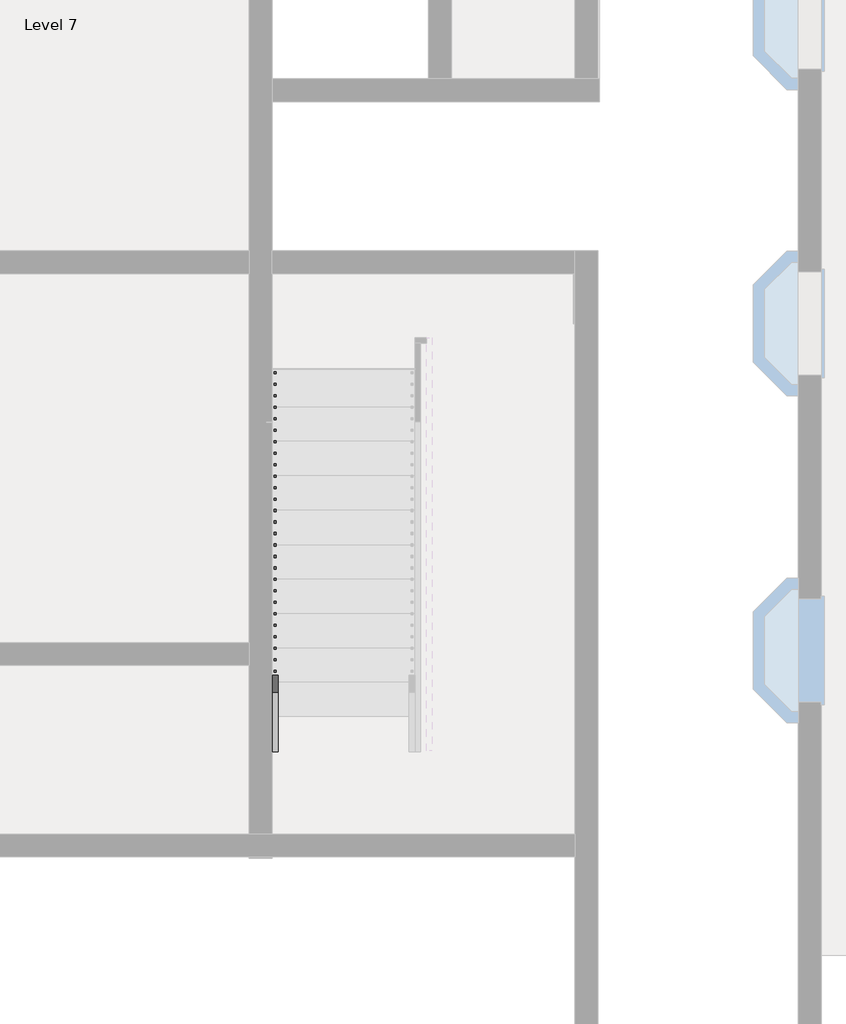
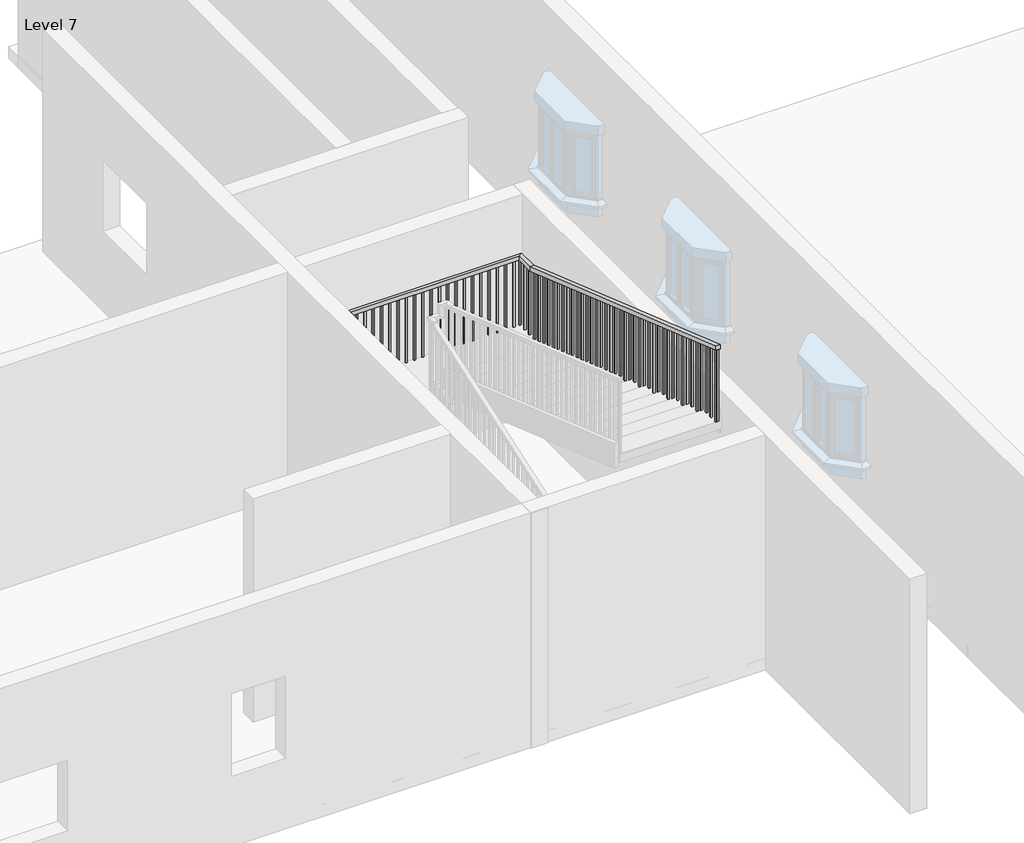
# One storey, part 8 of 14: 1 railing.
"""IFC4 building model written with IfcOpenShell, lengths in millimetres."""

from ifc_helpers import new_model, si_unit, frame, origin, place, context, project, spatial, polyline, outline, extrude, faceted_brep, element, save

model = new_model("IFC4")

# Units and contexts
model_context = context("Model", 3, world=origin())
ifc_project = project(units=[si_unit("LENGTHUNIT", "METRE", prefix="MILLI")], contexts=[model_context])

# Site, building, storey
site = spatial("IfcSite", under=ifc_project)
building = spatial("IfcBuilding", under=site)
storey = spatial("IfcBuildingStorey", under=building, Name="Level 7", Elevation=18288.0)

# Railing
placement = place(None, origin())
element("IfcRailing", 1, ObjectType="Handrail - Rectangular", at=placement, inside=storey, context=model_context, shape_type="SolidModel", body=[
    faceted_brep([(-3857.687215, -9955.5916506, 19307.9076923), (-3857.687215, -9955.5916506, 19254.1602476), (-3806.887215, -9955.5916506, 19254.1602476), (-3806.887215, -9955.5916506, 19307.9076923), (-3857.687215, -6291.6416506, 20574.0), (-3857.687215, -6283.1120276, 20523.2), (-3806.887215, -6283.1120276, 20523.2), (-3806.887215, -6291.6416506, 20574.0), (-3857.687215, -5713.7916506, 20574.0), (-3857.687215, -5713.7916506, 20523.2), (-3806.887215, -5764.5916506, 20523.2), (-3806.887215, -5764.5916506, 20574.0), (-1190.687215, -5713.7916506, 20574.0), (-1190.687215, -5713.7916506, 20523.2), (-1241.487215, -5764.5916506, 20523.2), (-1241.487215, -5764.5916506, 20574.0), (-1190.687215, -5986.8416506, 20574.0), (-1190.687215, -5995.3852679, 20523.2), (-1241.487215, -5995.3852679, 20523.2), (-1241.487215, -5986.8416506, 20574.0), (-1190.687215, -9949.2416506, 21945.6), (-1241.487215, -9949.2416506, 21945.6), (-1241.487215, -9949.2416506, 21891.842594), (-1190.687215, -9949.2416506, 21891.842594)], [[[0, 1, 2, 3]], [[1, 0, 4, 5]], [[2, 1, 5, 6]], [[3, 2, 6, 7]], [[0, 3, 7, 4]], [[5, 4, 8, 9]], [[6, 5, 9, 10]], [[7, 6, 10, 11]], [[4, 7, 11, 8]], [[9, 8, 12, 13]], [[10, 9, 13, 14]], [[11, 10, 14, 15]], [[8, 11, 15, 12]], [[13, 12, 16, 17]], [[14, 13, 17, 18]], [[15, 14, 18, 19]], [[12, 15, 19, 16]], [[20, 21, 22, 23]], [[17, 16, 20, 23]], [[18, 17, 23, 22]], [[19, 18, 22, 21]], [[16, 19, 21, 20]]]),
    extrude(outline(polyline([(-9895.2666506, 21873.1589402), (-9895.2666506, 20925.6923077), (-9914.3166506, 20925.6923077), (-9914.3166506, 21879.7531709), (-9895.2666506, 21873.1589402)])), frame((-1225.612215, 0.0, 0.0), z_axis=(1.0, 0.0, 0.0), x_axis=(0.0, 1.0, 0.0)), (0.0, 0.0, 1.0), 19.05),
    extrude(outline(polyline([(-9793.6666506, 21837.9897094), (-9793.6666506, 20925.6923077), (-9812.7166506, 20925.6923077), (-9812.7166506, 21844.5839402), (-9793.6666506, 21837.9897094)])), frame((-1225.612215, 0.0, 0.0), z_axis=(1.0, 0.0, 0.0), x_axis=(0.0, 1.0, 0.0)), (0.0, 0.0, 1.0), 19.05),
    extrude(outline(polyline([(-9692.0666506, 21802.8204786), (-9692.0666506, 20925.6923077), (-9711.1166506, 20925.6923077), (-9711.1166506, 21809.4147094), (-9692.0666506, 21802.8204786)])), frame((-1225.612215, 0.0, 0.0), z_axis=(1.0, 0.0, 0.0), x_axis=(0.0, 1.0, 0.0)), (0.0, 0.0, 1.0), 19.05),
    extrude(outline(polyline([(-9590.4666506, 21767.6512479), (-9590.4666506, 20820.1846154), (-9609.5166506, 20820.1846154), (-9609.5166506, 21774.2454786), (-9590.4666506, 21767.6512479)])), frame((-1225.612215, 0.0, 0.0), z_axis=(1.0, 0.0, 0.0), x_axis=(0.0, 1.0, 0.0)), (0.0, 0.0, 1.0), 19.05),
    extrude(outline(polyline([(-9488.8666506, 21732.4820171), (-9488.8666506, 20820.1846154), (-9507.9166506, 20820.1846154), (-9507.9166506, 21739.0762479), (-9488.8666506, 21732.4820171)])), frame((-1225.612215, 0.0, 0.0), z_axis=(1.0, 0.0, 0.0), x_axis=(0.0, 1.0, 0.0)), (0.0, 0.0, 1.0), 19.05),
    extrude(outline(polyline([(-9387.2666506, 21697.3127863), (-9387.2666506, 20820.1846154), (-9406.3166506, 20820.1846154), (-9406.3166506, 21703.9070171), (-9387.2666506, 21697.3127863)])), frame((-1225.612215, 0.0, 0.0), z_axis=(1.0, 0.0, 0.0), x_axis=(0.0, 1.0, 0.0)), (0.0, 0.0, 1.0), 19.05),
    extrude(outline(polyline([(-9285.6666506, 21662.1435556), (-9285.6666506, 20714.6769231), (-9304.7166506, 20714.6769231), (-9304.7166506, 21668.7377863), (-9285.6666506, 21662.1435556)])), frame((-1225.612215, 0.0, 0.0), z_axis=(1.0, 0.0, 0.0), x_axis=(0.0, 1.0, 0.0)), (0.0, 0.0, 1.0), 19.05),
    extrude(outline(polyline([(-9184.0666506, 21626.9743248), (-9184.0666506, 20714.6769231), (-9203.1166506, 20714.6769231), (-9203.1166506, 21633.5685556), (-9184.0666506, 21626.9743248)])), frame((-1225.612215, 0.0, 0.0), z_axis=(1.0, 0.0, 0.0), x_axis=(0.0, 1.0, 0.0)), (0.0, 0.0, 1.0), 19.05),
    extrude(outline(polyline([(-9082.4666506, 21591.805094), (-9082.4666506, 20714.6769231), (-9101.5166506, 20714.6769231), (-9101.5166506, 21598.3993248), (-9082.4666506, 21591.805094)])), frame((-1225.612215, 0.0, 0.0), z_axis=(1.0, 0.0, 0.0), x_axis=(0.0, 1.0, 0.0)), (0.0, 0.0, 1.0), 19.05),
    extrude(outline(polyline([(-8980.8666506, 21556.6358632), (-8980.8666506, 20609.1692308), (-8999.9166506, 20609.1692308), (-8999.9166506, 21563.230094), (-8980.8666506, 21556.6358632)])), frame((-1225.612215, 0.0, 0.0), z_axis=(1.0, 0.0, 0.0), x_axis=(0.0, 1.0, 0.0)), (0.0, 0.0, 1.0), 19.05),
    extrude(outline(polyline([(-8879.2666506, 21521.4666325), (-8879.2666506, 20609.1692308), (-8898.3166506, 20609.1692308), (-8898.3166506, 21528.0608632), (-8879.2666506, 21521.4666325)])), frame((-1225.612215, 0.0, 0.0), z_axis=(1.0, 0.0, 0.0), x_axis=(0.0, 1.0, 0.0)), (0.0, 0.0, 1.0), 19.05),
    extrude(outline(polyline([(-8777.6666506, 21486.2974017), (-8777.6666506, 20609.1692308), (-8796.7166506, 20609.1692308), (-8796.7166506, 21492.8916325), (-8777.6666506, 21486.2974017)])), frame((-1225.612215, 0.0, 0.0), z_axis=(1.0, 0.0, 0.0), x_axis=(0.0, 1.0, 0.0)), (0.0, 0.0, 1.0), 19.05),
    extrude(outline(polyline([(-8676.0666506, 21451.1281709), (-8676.0666506, 20503.6615385), (-8695.1166506, 20503.6615385), (-8695.1166506, 21457.7224017), (-8676.0666506, 21451.1281709)])), frame((-1225.612215, 0.0, 0.0), z_axis=(1.0, 0.0, 0.0), x_axis=(0.0, 1.0, 0.0)), (0.0, 0.0, 1.0), 19.05),
    extrude(outline(polyline([(-8574.4666506, 21415.9589402), (-8574.4666506, 20503.6615385), (-8593.5166506, 20503.6615385), (-8593.5166506, 21422.5531709), (-8574.4666506, 21415.9589402)])), frame((-1225.612215, 0.0, 0.0), z_axis=(1.0, 0.0, 0.0), x_axis=(0.0, 1.0, 0.0)), (0.0, 0.0, 1.0), 19.05),
    extrude(outline(polyline([(-8472.8666506, 21380.7897094), (-8472.8666506, 20503.6615385), (-8491.9166506, 20503.6615385), (-8491.9166506, 21387.3839402), (-8472.8666506, 21380.7897094)])), frame((-1225.612215, 0.0, 0.0), z_axis=(1.0, 0.0, 0.0), x_axis=(0.0, 1.0, 0.0)), (0.0, 0.0, 1.0), 19.05),
    extrude(outline(polyline([(-8371.2666506, 21345.6204786), (-8371.2666506, 20398.1538462), (-8390.3166506, 20398.1538462), (-8390.3166506, 21352.2147094), (-8371.2666506, 21345.6204786)])), frame((-1225.612215, 0.0, 0.0), z_axis=(1.0, 0.0, 0.0), x_axis=(0.0, 1.0, 0.0)), (0.0, 0.0, 1.0), 19.05),
    extrude(outline(polyline([(-8269.6666506, 21310.4512479), (-8269.6666506, 20398.1538462), (-8288.7166506, 20398.1538462), (-8288.7166506, 21317.0454786), (-8269.6666506, 21310.4512479)])), frame((-1225.612215, 0.0, 0.0), z_axis=(1.0, 0.0, 0.0), x_axis=(0.0, 1.0, 0.0)), (0.0, 0.0, 1.0), 19.05),
    extrude(outline(polyline([(-8168.0666506, 21275.2820171), (-8168.0666506, 20398.1538462), (-8187.1166506, 20398.1538462), (-8187.1166506, 21281.8762479), (-8168.0666506, 21275.2820171)])), frame((-1225.612215, 0.0, 0.0), z_axis=(1.0, 0.0, 0.0), x_axis=(0.0, 1.0, 0.0)), (0.0, 0.0, 1.0), 19.05),
    extrude(outline(polyline([(-8066.4666506, 21240.1127863), (-8066.4666506, 20292.6461538), (-8085.5166506, 20292.6461538), (-8085.5166506, 21246.7070171), (-8066.4666506, 21240.1127863)])), frame((-1225.612215, 0.0, 0.0), z_axis=(1.0, 0.0, 0.0), x_axis=(0.0, 1.0, 0.0)), (0.0, 0.0, 1.0), 19.05),
    extrude(outline(polyline([(-7964.8666506, 21204.9435556), (-7964.8666506, 20292.6461538), (-7983.9166506, 20292.6461538), (-7983.9166506, 21211.5377863), (-7964.8666506, 21204.9435556)])), frame((-1225.612215, 0.0, 0.0), z_axis=(1.0, 0.0, 0.0), x_axis=(0.0, 1.0, 0.0)), (0.0, 0.0, 1.0), 19.05),
    extrude(outline(polyline([(-7863.2666506, 21169.7743248), (-7863.2666506, 20292.6461538), (-7882.3166506, 20292.6461538), (-7882.3166506, 21176.3685556), (-7863.2666506, 21169.7743248)])), frame((-1225.612215, 0.0, 0.0), z_axis=(1.0, 0.0, 0.0), x_axis=(0.0, 1.0, 0.0)), (0.0, 0.0, 1.0), 19.05),
    extrude(outline(polyline([(-7761.6666506, 21134.605094), (-7761.6666506, 20187.1384615), (-7780.7166506, 20187.1384615), (-7780.7166506, 21141.1993248), (-7761.6666506, 21134.605094)])), frame((-1225.612215, 0.0, 0.0), z_axis=(1.0, 0.0, 0.0), x_axis=(0.0, 1.0, 0.0)), (0.0, 0.0, 1.0), 19.05),
    extrude(outline(polyline([(-7660.0666506, 21099.4358632), (-7660.0666506, 20187.1384615), (-7679.1166506, 20187.1384615), (-7679.1166506, 21106.030094), (-7660.0666506, 21099.4358632)])), frame((-1225.612215, 0.0, 0.0), z_axis=(1.0, 0.0, 0.0), x_axis=(0.0, 1.0, 0.0)), (0.0, 0.0, 1.0), 19.05),
    extrude(outline(polyline([(-7558.4666506, 21064.2666325), (-7558.4666506, 20187.1384615), (-7577.5166506, 20187.1384615), (-7577.5166506, 21070.8608632), (-7558.4666506, 21064.2666325)])), frame((-1225.612215, 0.0, 0.0), z_axis=(1.0, 0.0, 0.0), x_axis=(0.0, 1.0, 0.0)), (0.0, 0.0, 1.0), 19.05),
    extrude(outline(polyline([(-7456.8666506, 21029.0974017), (-7456.8666506, 20081.6307692), (-7475.9166506, 20081.6307692), (-7475.9166506, 21035.6916325), (-7456.8666506, 21029.0974017)])), frame((-1225.612215, 0.0, 0.0), z_axis=(1.0, 0.0, 0.0), x_axis=(0.0, 1.0, 0.0)), (0.0, 0.0, 1.0), 19.05),
    extrude(outline(polyline([(-7355.2666506, 20993.9281709), (-7355.2666506, 20081.6307692), (-7374.3166506, 20081.6307692), (-7374.3166506, 21000.5224017), (-7355.2666506, 20993.9281709)])), frame((-1225.612215, 0.0, 0.0), z_axis=(1.0, 0.0, 0.0), x_axis=(0.0, 1.0, 0.0)), (0.0, 0.0, 1.0), 19.05),
    extrude(outline(polyline([(-7253.6666506, 20958.7589402), (-7253.6666506, 20081.6307692), (-7272.7166506, 20081.6307692), (-7272.7166506, 20965.3531709), (-7253.6666506, 20958.7589402)])), frame((-1225.612215, 0.0, 0.0), z_axis=(1.0, 0.0, 0.0), x_axis=(0.0, 1.0, 0.0)), (0.0, 0.0, 1.0), 19.05),
    extrude(outline(polyline([(-7152.0666506, 20923.5897094), (-7152.0666506, 19976.1230769), (-7171.1166506, 19976.1230769), (-7171.1166506, 20930.1839402), (-7152.0666506, 20923.5897094)])), frame((-1225.612215, 0.0, 0.0), z_axis=(1.0, 0.0, 0.0), x_axis=(0.0, 1.0, 0.0)), (0.0, 0.0, 1.0), 19.05),
    extrude(outline(polyline([(-7050.4666506, 20888.4204786), (-7050.4666506, 19976.1230769), (-7069.5166506, 19976.1230769), (-7069.5166506, 20895.0147094), (-7050.4666506, 20888.4204786)])), frame((-1225.612215, 0.0, 0.0), z_axis=(1.0, 0.0, 0.0), x_axis=(0.0, 1.0, 0.0)), (0.0, 0.0, 1.0), 19.05),
    extrude(outline(polyline([(-6948.8666506, 20853.2512479), (-6948.8666506, 19976.1230769), (-6967.9166506, 19976.1230769), (-6967.9166506, 20859.8454786), (-6948.8666506, 20853.2512479)])), frame((-1225.612215, 0.0, 0.0), z_axis=(1.0, 0.0, 0.0), x_axis=(0.0, 1.0, 0.0)), (0.0, 0.0, 1.0), 19.05),
    extrude(outline(polyline([(-6847.2666506, 20818.0820171), (-6847.2666506, 19870.6153846), (-6866.3166506, 19870.6153846), (-6866.3166506, 20824.6762479), (-6847.2666506, 20818.0820171)])), frame((-1225.612215, 0.0, 0.0), z_axis=(1.0, 0.0, 0.0), x_axis=(0.0, 1.0, 0.0)), (0.0, 0.0, 1.0), 19.05),
    extrude(outline(polyline([(-6745.6666506, 20782.9127863), (-6745.6666506, 19870.6153846), (-6764.7166506, 19870.6153846), (-6764.7166506, 20789.5070171), (-6745.6666506, 20782.9127863)])), frame((-1225.612215, 0.0, 0.0), z_axis=(1.0, 0.0, 0.0), x_axis=(0.0, 1.0, 0.0)), (0.0, 0.0, 1.0), 19.05),
    extrude(outline(polyline([(-6644.0666506, 20747.7435556), (-6644.0666506, 19870.6153846), (-6663.1166506, 19870.6153846), (-6663.1166506, 20754.3377863), (-6644.0666506, 20747.7435556)])), frame((-1225.612215, 0.0, 0.0), z_axis=(1.0, 0.0, 0.0), x_axis=(0.0, 1.0, 0.0)), (0.0, 0.0, 1.0), 19.05),
    extrude(outline(polyline([(-6542.4666506, 20712.5743248), (-6542.4666506, 19765.1076923), (-6561.5166506, 19765.1076923), (-6561.5166506, 20719.1685556), (-6542.4666506, 20712.5743248)])), frame((-1225.612215, 0.0, 0.0), z_axis=(1.0, 0.0, 0.0), x_axis=(0.0, 1.0, 0.0)), (0.0, 0.0, 1.0), 19.05),
    extrude(outline(polyline([(-6440.8666506, 20677.405094), (-6440.8666506, 19765.1076923), (-6459.9166506, 19765.1076923), (-6459.9166506, 20683.9993248), (-6440.8666506, 20677.405094)])), frame((-1225.612215, 0.0, 0.0), z_axis=(1.0, 0.0, 0.0), x_axis=(0.0, 1.0, 0.0)), (0.0, 0.0, 1.0), 19.05),
    extrude(outline(polyline([(-6339.2666506, 20642.2358632), (-6339.2666506, 19765.1076923), (-6358.3166506, 19765.1076923), (-6358.3166506, 20648.830094), (-6339.2666506, 20642.2358632)])), frame((-1225.612215, 0.0, 0.0), z_axis=(1.0, 0.0, 0.0), x_axis=(0.0, 1.0, 0.0)), (0.0, 0.0, 1.0), 19.05),
    extrude(outline(polyline([(-6237.6666506, 20607.0666325), (-6237.6666506, 19659.6), (-6256.7166506, 19659.6), (-6256.7166506, 20613.6608632), (-6237.6666506, 20607.0666325)])), frame((-1225.612215, 0.0, 0.0), z_axis=(1.0, 0.0, 0.0), x_axis=(0.0, 1.0, 0.0)), (0.0, 0.0, 1.0), 19.05),
    extrude(outline(polyline([(-6136.0666506, 20571.8974017), (-6136.0666506, 19659.6), (-6155.1166506, 19659.6), (-6155.1166506, 20578.4916325), (-6136.0666506, 20571.8974017)])), frame((-1225.612215, 0.0, 0.0), z_axis=(1.0, 0.0, 0.0), x_axis=(0.0, 1.0, 0.0)), (0.0, 0.0, 1.0), 19.05),
    extrude(outline(polyline([(-6034.4666506, 20536.7281709), (-6034.4666506, 19659.6), (-6053.5166506, 19659.6), (-6053.5166506, 20543.3224017), (-6034.4666506, 20536.7281709)])), frame((-1225.612215, 0.0, 0.0), z_axis=(1.0, 0.0, 0.0), x_axis=(0.0, 1.0, 0.0)), (0.0, 0.0, 1.0), 19.05),
    extrude(outline(polyline([(-1206.562215, -5932.8666506), (-1206.562215, -5951.9166506), (-1225.612215, -5951.9166506), (-1225.612215, -5932.8666506), (-1206.562215, -5932.8666506)])), frame((0.0, 0.0, 19659.6), z_axis=(0.0, 0.0, 1.0), x_axis=(1.0, 0.0, 0.0)), (0.0, 0.0, 1.0), 863.6),
    extrude(outline(polyline([(-1206.562215, -5831.2666506), (-1206.562215, -5850.3166506), (-1225.612215, -5850.3166506), (-1225.612215, -5831.2666506), (-1206.562215, -5831.2666506)])), frame((0.0, 0.0, 19659.6), z_axis=(0.0, 0.0, 1.0), x_axis=(1.0, 0.0, 0.0)), (0.0, 0.0, 1.0), 863.6),
    extrude(outline(polyline([(-1301.812215, -5729.6666506), (-1282.762215, -5729.6666506), (-1282.762215, -5748.7166506), (-1301.812215, -5748.7166506), (-1301.812215, -5729.6666506)])), frame((0.0, 0.0, 19659.6), z_axis=(0.0, 0.0, 1.0), x_axis=(1.0, 0.0, 0.0)), (0.0, 0.0, 1.0), 863.6),
    extrude(outline(polyline([(-1403.412215, -5729.6666506), (-1384.362215, -5729.6666506), (-1384.362215, -5748.7166506), (-1403.412215, -5748.7166506), (-1403.412215, -5729.6666506)])), frame((0.0, 0.0, 19659.6), z_axis=(0.0, 0.0, 1.0), x_axis=(1.0, 0.0, 0.0)), (0.0, 0.0, 1.0), 863.6),
    extrude(outline(polyline([(-1505.012215, -5729.6666506), (-1485.962215, -5729.6666506), (-1485.962215, -5748.7166506), (-1505.012215, -5748.7166506), (-1505.012215, -5729.6666506)])), frame((0.0, 0.0, 19659.6), z_axis=(0.0, 0.0, 1.0), x_axis=(1.0, 0.0, 0.0)), (0.0, 0.0, 1.0), 863.6),
    extrude(outline(polyline([(-1606.612215, -5729.6666506), (-1587.562215, -5729.6666506), (-1587.562215, -5748.7166506), (-1606.612215, -5748.7166506), (-1606.612215, -5729.6666506)])), frame((0.0, 0.0, 19659.6), z_axis=(0.0, 0.0, 1.0), x_axis=(1.0, 0.0, 0.0)), (0.0, 0.0, 1.0), 863.6),
    extrude(outline(polyline([(-1708.212215, -5729.6666506), (-1689.162215, -5729.6666506), (-1689.162215, -5748.7166506), (-1708.212215, -5748.7166506), (-1708.212215, -5729.6666506)])), frame((0.0, 0.0, 19659.6), z_axis=(0.0, 0.0, 1.0), x_axis=(1.0, 0.0, 0.0)), (0.0, 0.0, 1.0), 863.6),
    extrude(outline(polyline([(-1809.812215, -5729.6666506), (-1790.762215, -5729.6666506), (-1790.762215, -5748.7166506), (-1809.812215, -5748.7166506), (-1809.812215, -5729.6666506)])), frame((0.0, 0.0, 19659.6), z_axis=(0.0, 0.0, 1.0), x_axis=(1.0, 0.0, 0.0)), (0.0, 0.0, 1.0), 863.6),
    extrude(outline(polyline([(-1911.412215, -5729.6666506), (-1892.362215, -5729.6666506), (-1892.362215, -5748.7166506), (-1911.412215, -5748.7166506), (-1911.412215, -5729.6666506)])), frame((0.0, 0.0, 19659.6), z_axis=(0.0, 0.0, 1.0), x_axis=(1.0, 0.0, 0.0)), (0.0, 0.0, 1.0), 863.6),
    extrude(outline(polyline([(-2013.012215, -5729.6666506), (-1993.962215, -5729.6666506), (-1993.962215, -5748.7166506), (-2013.012215, -5748.7166506), (-2013.012215, -5729.6666506)])), frame((0.0, 0.0, 19659.6), z_axis=(0.0, 0.0, 1.0), x_axis=(1.0, 0.0, 0.0)), (0.0, 0.0, 1.0), 863.6),
    extrude(outline(polyline([(-2114.612215, -5729.6666506), (-2095.562215, -5729.6666506), (-2095.562215, -5748.7166506), (-2114.612215, -5748.7166506), (-2114.612215, -5729.6666506)])), frame((0.0, 0.0, 19659.6), z_axis=(0.0, 0.0, 1.0), x_axis=(1.0, 0.0, 0.0)), (0.0, 0.0, 1.0), 863.6),
    extrude(outline(polyline([(-2216.212215, -5729.6666506), (-2197.162215, -5729.6666506), (-2197.162215, -5748.7166506), (-2216.212215, -5748.7166506), (-2216.212215, -5729.6666506)])), frame((0.0, 0.0, 19659.6), z_axis=(0.0, 0.0, 1.0), x_axis=(1.0, 0.0, 0.0)), (0.0, 0.0, 1.0), 863.6),
    extrude(outline(polyline([(-2317.812215, -5729.6666506), (-2298.762215, -5729.6666506), (-2298.762215, -5748.7166506), (-2317.812215, -5748.7166506), (-2317.812215, -5729.6666506)])), frame((0.0, 0.0, 19659.6), z_axis=(0.0, 0.0, 1.0), x_axis=(1.0, 0.0, 0.0)), (0.0, 0.0, 1.0), 863.6),
    extrude(outline(polyline([(-2419.412215, -5729.6666506), (-2400.362215, -5729.6666506), (-2400.362215, -5748.7166506), (-2419.412215, -5748.7166506), (-2419.412215, -5729.6666506)])), frame((0.0, 0.0, 19659.6), z_axis=(0.0, 0.0, 1.0), x_axis=(1.0, 0.0, 0.0)), (0.0, 0.0, 1.0), 863.6),
    extrude(outline(polyline([(-2521.012215, -5729.6666506), (-2501.962215, -5729.6666506), (-2501.962215, -5748.7166506), (-2521.012215, -5748.7166506), (-2521.012215, -5729.6666506)])), frame((0.0, 0.0, 19659.6), z_axis=(0.0, 0.0, 1.0), x_axis=(1.0, 0.0, 0.0)), (0.0, 0.0, 1.0), 863.6),
    extrude(outline(polyline([(-2622.612215, -5729.6666506), (-2603.562215, -5729.6666506), (-2603.562215, -5748.7166506), (-2622.612215, -5748.7166506), (-2622.612215, -5729.6666506)])), frame((0.0, 0.0, 19659.6), z_axis=(0.0, 0.0, 1.0), x_axis=(1.0, 0.0, 0.0)), (0.0, 0.0, 1.0), 863.6),
    extrude(outline(polyline([(-2724.212215, -5729.6666506), (-2705.162215, -5729.6666506), (-2705.162215, -5748.7166506), (-2724.212215, -5748.7166506), (-2724.212215, -5729.6666506)])), frame((0.0, 0.0, 19659.6), z_axis=(0.0, 0.0, 1.0), x_axis=(1.0, 0.0, 0.0)), (0.0, 0.0, 1.0), 863.6),
    extrude(outline(polyline([(-2825.812215, -5729.6666506), (-2806.762215, -5729.6666506), (-2806.762215, -5748.7166506), (-2825.812215, -5748.7166506), (-2825.812215, -5729.6666506)])), frame((0.0, 0.0, 19659.6), z_axis=(0.0, 0.0, 1.0), x_axis=(1.0, 0.0, 0.0)), (0.0, 0.0, 1.0), 863.6),
    extrude(outline(polyline([(-2927.412215, -5729.6666506), (-2908.362215, -5729.6666506), (-2908.362215, -5748.7166506), (-2927.412215, -5748.7166506), (-2927.412215, -5729.6666506)])), frame((0.0, 0.0, 19659.6), z_axis=(0.0, 0.0, 1.0), x_axis=(1.0, 0.0, 0.0)), (0.0, 0.0, 1.0), 863.6),
    extrude(outline(polyline([(-3029.012215, -5729.6666506), (-3009.962215, -5729.6666506), (-3009.962215, -5748.7166506), (-3029.012215, -5748.7166506), (-3029.012215, -5729.6666506)])), frame((0.0, 0.0, 19659.6), z_axis=(0.0, 0.0, 1.0), x_axis=(1.0, 0.0, 0.0)), (0.0, 0.0, 1.0), 863.6),
    extrude(outline(polyline([(-3130.612215, -5729.6666506), (-3111.562215, -5729.6666506), (-3111.562215, -5748.7166506), (-3130.612215, -5748.7166506), (-3130.612215, -5729.6666506)])), frame((0.0, 0.0, 19659.6), z_axis=(0.0, 0.0, 1.0), x_axis=(1.0, 0.0, 0.0)), (0.0, 0.0, 1.0), 863.6),
    extrude(outline(polyline([(-3232.212215, -5729.6666506), (-3213.162215, -5729.6666506), (-3213.162215, -5748.7166506), (-3232.212215, -5748.7166506), (-3232.212215, -5729.6666506)])), frame((0.0, 0.0, 19659.6), z_axis=(0.0, 0.0, 1.0), x_axis=(1.0, 0.0, 0.0)), (0.0, 0.0, 1.0), 863.6),
    extrude(outline(polyline([(-3333.812215, -5729.6666506), (-3314.762215, -5729.6666506), (-3314.762215, -5748.7166506), (-3333.812215, -5748.7166506), (-3333.812215, -5729.6666506)])), frame((0.0, 0.0, 19659.6), z_axis=(0.0, 0.0, 1.0), x_axis=(1.0, 0.0, 0.0)), (0.0, 0.0, 1.0), 863.6),
    extrude(outline(polyline([(-3435.412215, -5729.6666506), (-3416.362215, -5729.6666506), (-3416.362215, -5748.7166506), (-3435.412215, -5748.7166506), (-3435.412215, -5729.6666506)])), frame((0.0, 0.0, 19659.6), z_axis=(0.0, 0.0, 1.0), x_axis=(1.0, 0.0, 0.0)), (0.0, 0.0, 1.0), 863.6),
    extrude(outline(polyline([(-3537.012215, -5729.6666506), (-3517.962215, -5729.6666506), (-3517.962215, -5748.7166506), (-3537.012215, -5748.7166506), (-3537.012215, -5729.6666506)])), frame((0.0, 0.0, 19659.6), z_axis=(0.0, 0.0, 1.0), x_axis=(1.0, 0.0, 0.0)), (0.0, 0.0, 1.0), 863.6),
    extrude(outline(polyline([(-3638.612215, -5729.6666506), (-3619.562215, -5729.6666506), (-3619.562215, -5748.7166506), (-3638.612215, -5748.7166506), (-3638.612215, -5729.6666506)])), frame((0.0, 0.0, 19659.6), z_axis=(0.0, 0.0, 1.0), x_axis=(1.0, 0.0, 0.0)), (0.0, 0.0, 1.0), 863.6),
    extrude(outline(polyline([(-3740.212215, -5729.6666506), (-3721.162215, -5729.6666506), (-3721.162215, -5748.7166506), (-3740.212215, -5748.7166506), (-3740.212215, -5729.6666506)])), frame((0.0, 0.0, 19659.6), z_axis=(0.0, 0.0, 1.0), x_axis=(1.0, 0.0, 0.0)), (0.0, 0.0, 1.0), 863.6),
    extrude(outline(polyline([(-3841.812215, -5799.5166506), (-3841.812215, -5780.4666506), (-3822.762215, -5780.4666506), (-3822.762215, -5799.5166506), (-3841.812215, -5799.5166506)])), frame((0.0, 0.0, 19659.6), z_axis=(0.0, 0.0, 1.0), x_axis=(1.0, 0.0, 0.0)), (0.0, 0.0, 1.0), 863.6),
    extrude(outline(polyline([(-3841.812215, -5901.1166506), (-3841.812215, -5882.0666506), (-3822.762215, -5882.0666506), (-3822.762215, -5901.1166506), (-3841.812215, -5901.1166506)])), frame((0.0, 0.0, 19659.6), z_axis=(0.0, 0.0, 1.0), x_axis=(1.0, 0.0, 0.0)), (0.0, 0.0, 1.0), 863.6),
    extrude(outline(polyline([(-3841.812215, -6002.7166506), (-3841.812215, -5983.6666506), (-3822.762215, -5983.6666506), (-3822.762215, -6002.7166506), (-3841.812215, -6002.7166506)])), frame((0.0, 0.0, 19659.6), z_axis=(0.0, 0.0, 1.0), x_axis=(1.0, 0.0, 0.0)), (0.0, 0.0, 1.0), 863.6),
    extrude(outline(polyline([(-3841.812215, -6104.3166506), (-3841.812215, -6085.2666506), (-3822.762215, -6085.2666506), (-3822.762215, -6104.3166506), (-3841.812215, -6104.3166506)])), frame((0.0, 0.0, 19659.6), z_axis=(0.0, 0.0, 1.0), x_axis=(1.0, 0.0, 0.0)), (0.0, 0.0, 1.0), 863.6),
    extrude(outline(polyline([(-3841.812215, -6205.9166506), (-3841.812215, -6186.8666506), (-3822.762215, -6186.8666506), (-3822.762215, -6205.9166506), (-3841.812215, -6205.9166506)])), frame((0.0, 0.0, 19659.6), z_axis=(0.0, 0.0, 1.0), x_axis=(1.0, 0.0, 0.0)), (0.0, 0.0, 1.0), 863.6),
    extrude(outline(polyline([(-6288.4666506, 20521.349689), (-6288.4666506, 19554.0923077), (-6307.5166506, 19554.0923077), (-6307.5166506, 20514.7668867), (-6288.4666506, 20521.349689)])), frame((-3841.812215, 0.0, 0.0), z_axis=(1.0, 0.0, 0.0), x_axis=(0.0, 1.0, 0.0)), (0.0, 0.0, 1.0), 19.05),
    extrude(outline(polyline([(-6390.0666506, 20486.2414101), (-6390.0666506, 19554.0923077), (-6409.1166506, 19554.0923077), (-6409.1166506, 20479.6586078), (-6390.0666506, 20486.2414101)])), frame((-3841.812215, 0.0, 0.0), z_axis=(1.0, 0.0, 0.0), x_axis=(0.0, 1.0, 0.0)), (0.0, 0.0, 1.0), 19.05),
    extrude(outline(polyline([(-6491.6666506, 20451.1331312), (-6491.6666506, 19554.0923077), (-6510.7166506, 19554.0923077), (-6510.7166506, 20444.5503289), (-6491.6666506, 20451.1331312)])), frame((-3841.812215, 0.0, 0.0), z_axis=(1.0, 0.0, 0.0), x_axis=(0.0, 1.0, 0.0)), (0.0, 0.0, 1.0), 19.05),
    extrude(outline(polyline([(-6593.2666506, 20416.0248523), (-6593.2666506, 19448.5846154), (-6612.3166506, 19448.5846154), (-6612.3166506, 20409.44205), (-6593.2666506, 20416.0248523)])), frame((-3841.812215, 0.0, 0.0), z_axis=(1.0, 0.0, 0.0), x_axis=(0.0, 1.0, 0.0)), (0.0, 0.0, 1.0), 19.05),
    extrude(outline(polyline([(-6694.8666506, 20380.9165734), (-6694.8666506, 19448.5846154), (-6713.9166506, 19448.5846154), (-6713.9166506, 20374.3337711), (-6694.8666506, 20380.9165734)])), frame((-3841.812215, 0.0, 0.0), z_axis=(1.0, 0.0, 0.0), x_axis=(0.0, 1.0, 0.0)), (0.0, 0.0, 1.0), 19.05),
    extrude(outline(polyline([(-6796.4666506, 20345.8082945), (-6796.4666506, 19448.5846154), (-6815.5166506, 19448.5846154), (-6815.5166506, 20339.2254922), (-6796.4666506, 20345.8082945)])), frame((-3841.812215, 0.0, 0.0), z_axis=(1.0, 0.0, 0.0), x_axis=(0.0, 1.0, 0.0)), (0.0, 0.0, 1.0), 19.05),
    extrude(outline(polyline([(-6898.0666506, 20310.7000156), (-6898.0666506, 19343.0769231), (-6917.1166506, 19343.0769231), (-6917.1166506, 20304.1172133), (-6898.0666506, 20310.7000156)])), frame((-3841.812215, 0.0, 0.0), z_axis=(1.0, 0.0, 0.0), x_axis=(0.0, 1.0, 0.0)), (0.0, 0.0, 1.0), 19.05),
    extrude(outline(polyline([(-6999.6666506, 20275.5917367), (-6999.6666506, 19343.0769231), (-7018.7166506, 19343.0769231), (-7018.7166506, 20269.0089344), (-6999.6666506, 20275.5917367)])), frame((-3841.812215, 0.0, 0.0), z_axis=(1.0, 0.0, 0.0), x_axis=(0.0, 1.0, 0.0)), (0.0, 0.0, 1.0), 19.05),
    extrude(outline(polyline([(-7101.2666506, 20240.4834578), (-7101.2666506, 19343.0769231), (-7120.3166506, 19343.0769231), (-7120.3166506, 20233.9006556), (-7101.2666506, 20240.4834578)])), frame((-3841.812215, 0.0, 0.0), z_axis=(1.0, 0.0, 0.0), x_axis=(0.0, 1.0, 0.0)), (0.0, 0.0, 1.0), 19.05),
    extrude(outline(polyline([(-7202.8666506, 20205.375179), (-7202.8666506, 19237.5692308), (-7221.9166506, 19237.5692308), (-7221.9166506, 20198.7923767), (-7202.8666506, 20205.375179)])), frame((-3841.812215, 0.0, 0.0), z_axis=(1.0, 0.0, 0.0), x_axis=(0.0, 1.0, 0.0)), (0.0, 0.0, 1.0), 19.05),
    extrude(outline(polyline([(-7304.4666506, 20170.2669001), (-7304.4666506, 19237.5692308), (-7323.5166506, 19237.5692308), (-7323.5166506, 20163.6840978), (-7304.4666506, 20170.2669001)])), frame((-3841.812215, 0.0, 0.0), z_axis=(1.0, 0.0, 0.0), x_axis=(0.0, 1.0, 0.0)), (0.0, 0.0, 1.0), 19.05),
    extrude(outline(polyline([(-7406.0666506, 20135.1586212), (-7406.0666506, 19237.5692308), (-7425.1166506, 19237.5692308), (-7425.1166506, 20128.5758189), (-7406.0666506, 20135.1586212)])), frame((-3841.812215, 0.0, 0.0), z_axis=(1.0, 0.0, 0.0), x_axis=(0.0, 1.0, 0.0)), (0.0, 0.0, 1.0), 19.05),
    extrude(outline(polyline([(-7507.6666506, 20100.0503423), (-7507.6666506, 19132.0615385), (-7526.7166506, 19132.0615385), (-7526.7166506, 20093.46754), (-7507.6666506, 20100.0503423)])), frame((-3841.812215, 0.0, 0.0), z_axis=(1.0, 0.0, 0.0), x_axis=(0.0, 1.0, 0.0)), (0.0, 0.0, 1.0), 19.05),
    extrude(outline(polyline([(-7609.2666506, 20064.9420634), (-7609.2666506, 19132.0615385), (-7628.3166506, 19132.0615385), (-7628.3166506, 20058.3592611), (-7609.2666506, 20064.9420634)])), frame((-3841.812215, 0.0, 0.0), z_axis=(1.0, 0.0, 0.0), x_axis=(0.0, 1.0, 0.0)), (0.0, 0.0, 1.0), 19.05),
    extrude(outline(polyline([(-7710.8666506, 20029.8337845), (-7710.8666506, 19132.0615385), (-7729.9166506, 19132.0615385), (-7729.9166506, 20023.2509822), (-7710.8666506, 20029.8337845)])), frame((-3841.812215, 0.0, 0.0), z_axis=(1.0, 0.0, 0.0), x_axis=(0.0, 1.0, 0.0)), (0.0, 0.0, 1.0), 19.05),
    extrude(outline(polyline([(-7812.4666506, 19994.7255056), (-7812.4666506, 19026.5538462), (-7831.5166506, 19026.5538462), (-7831.5166506, 19988.1427033), (-7812.4666506, 19994.7255056)])), frame((-3841.812215, 0.0, 0.0), z_axis=(1.0, 0.0, 0.0), x_axis=(0.0, 1.0, 0.0)), (0.0, 0.0, 1.0), 19.05),
    extrude(outline(polyline([(-7914.0666506, 19959.6172267), (-7914.0666506, 19026.5538462), (-7933.1166506, 19026.5538462), (-7933.1166506, 19953.0344244), (-7914.0666506, 19959.6172267)])), frame((-3841.812215, 0.0, 0.0), z_axis=(1.0, 0.0, 0.0), x_axis=(0.0, 1.0, 0.0)), (0.0, 0.0, 1.0), 19.05),
    extrude(outline(polyline([(-8015.6666506, 19924.5089478), (-8015.6666506, 19026.5538462), (-8034.7166506, 19026.5538462), (-8034.7166506, 19917.9261455), (-8015.6666506, 19924.5089478)])), frame((-3841.812215, 0.0, 0.0), z_axis=(1.0, 0.0, 0.0), x_axis=(0.0, 1.0, 0.0)), (0.0, 0.0, 1.0), 19.05),
    extrude(outline(polyline([(-8117.2666506, 19889.4006689), (-8117.2666506, 18921.0461538), (-8136.3166506, 18921.0461538), (-8136.3166506, 19882.8178666), (-8117.2666506, 19889.4006689)])), frame((-3841.812215, 0.0, 0.0), z_axis=(1.0, 0.0, 0.0), x_axis=(0.0, 1.0, 0.0)), (0.0, 0.0, 1.0), 19.05),
    extrude(outline(polyline([(-8218.8666506, 19854.29239), (-8218.8666506, 18921.0461538), (-8237.9166506, 18921.0461538), (-8237.9166506, 19847.7095877), (-8218.8666506, 19854.29239)])), frame((-3841.812215, 0.0, 0.0), z_axis=(1.0, 0.0, 0.0), x_axis=(0.0, 1.0, 0.0)), (0.0, 0.0, 1.0), 19.05),
    extrude(outline(polyline([(-8320.4666506, 19819.1841111), (-8320.4666506, 18921.0461538), (-8339.5166506, 18921.0461538), (-8339.5166506, 19812.6013088), (-8320.4666506, 19819.1841111)])), frame((-3841.812215, 0.0, 0.0), z_axis=(1.0, 0.0, 0.0), x_axis=(0.0, 1.0, 0.0)), (0.0, 0.0, 1.0), 19.05),
    extrude(outline(polyline([(-8422.0666506, 19784.0758322), (-8422.0666506, 18815.5384615), (-8441.1166506, 18815.5384615), (-8441.1166506, 19777.4930299), (-8422.0666506, 19784.0758322)])), frame((-3841.812215, 0.0, 0.0), z_axis=(1.0, 0.0, 0.0), x_axis=(0.0, 1.0, 0.0)), (0.0, 0.0, 1.0), 19.05),
    extrude(outline(polyline([(-8523.6666506, 19748.9675533), (-8523.6666506, 18815.5384615), (-8542.7166506, 18815.5384615), (-8542.7166506, 19742.384751), (-8523.6666506, 19748.9675533)])), frame((-3841.812215, 0.0, 0.0), z_axis=(1.0, 0.0, 0.0), x_axis=(0.0, 1.0, 0.0)), (0.0, 0.0, 1.0), 19.05),
    extrude(outline(polyline([(-8625.2666506, 19713.8592744), (-8625.2666506, 18815.5384615), (-8644.3166506, 18815.5384615), (-8644.3166506, 19707.2764721), (-8625.2666506, 19713.8592744)])), frame((-3841.812215, 0.0, 0.0), z_axis=(1.0, 0.0, 0.0), x_axis=(0.0, 1.0, 0.0)), (0.0, 0.0, 1.0), 19.05),
    extrude(outline(polyline([(-8726.8666506, 19678.7509955), (-8726.8666506, 18710.0307692), (-8745.9166506, 18710.0307692), (-8745.9166506, 19672.1681932), (-8726.8666506, 19678.7509955)])), frame((-3841.812215, 0.0, 0.0), z_axis=(1.0, 0.0, 0.0), x_axis=(0.0, 1.0, 0.0)), (0.0, 0.0, 1.0), 19.05),
    extrude(outline(polyline([(-8828.4666506, 19643.6427166), (-8828.4666506, 18710.0307692), (-8847.5166506, 18710.0307692), (-8847.5166506, 19637.0599143), (-8828.4666506, 19643.6427166)])), frame((-3841.812215, 0.0, 0.0), z_axis=(1.0, 0.0, 0.0), x_axis=(0.0, 1.0, 0.0)), (0.0, 0.0, 1.0), 19.05),
    extrude(outline(polyline([(-8930.0666506, 19608.5344377), (-8930.0666506, 18710.0307692), (-8949.1166506, 18710.0307692), (-8949.1166506, 19601.9516354), (-8930.0666506, 19608.5344377)])), frame((-3841.812215, 0.0, 0.0), z_axis=(1.0, 0.0, 0.0), x_axis=(0.0, 1.0, 0.0)), (0.0, 0.0, 1.0), 19.05),
    extrude(outline(polyline([(-9031.6666506, 19573.4261588), (-9031.6666506, 18604.5230769), (-9050.7166506, 18604.5230769), (-9050.7166506, 19566.8433565), (-9031.6666506, 19573.4261588)])), frame((-3841.812215, 0.0, 0.0), z_axis=(1.0, 0.0, 0.0), x_axis=(0.0, 1.0, 0.0)), (0.0, 0.0, 1.0), 19.05),
    extrude(outline(polyline([(-9133.2666506, 19538.3178799), (-9133.2666506, 18604.5230769), (-9152.3166506, 18604.5230769), (-9152.3166506, 19531.7350776), (-9133.2666506, 19538.3178799)])), frame((-3841.812215, 0.0, 0.0), z_axis=(1.0, 0.0, 0.0), x_axis=(0.0, 1.0, 0.0)), (0.0, 0.0, 1.0), 19.05),
    extrude(outline(polyline([(-9234.8666506, 19503.209601), (-9234.8666506, 18604.5230769), (-9253.9166506, 18604.5230769), (-9253.9166506, 19496.6267987), (-9234.8666506, 19503.209601)])), frame((-3841.812215, 0.0, 0.0), z_axis=(1.0, 0.0, 0.0), x_axis=(0.0, 1.0, 0.0)), (0.0, 0.0, 1.0), 19.05),
    extrude(outline(polyline([(-9336.4666506, 19468.1013221), (-9336.4666506, 18499.0153846), (-9355.5166506, 18499.0153846), (-9355.5166506, 19461.5185198), (-9336.4666506, 19468.1013221)])), frame((-3841.812215, 0.0, 0.0), z_axis=(1.0, 0.0, 0.0), x_axis=(0.0, 1.0, 0.0)), (0.0, 0.0, 1.0), 19.05),
    extrude(outline(polyline([(-9438.0666506, 19432.9930432), (-9438.0666506, 18499.0153846), (-9457.1166506, 18499.0153846), (-9457.1166506, 19426.4102409), (-9438.0666506, 19432.9930432)])), frame((-3841.812215, 0.0, 0.0), z_axis=(1.0, 0.0, 0.0), x_axis=(0.0, 1.0, 0.0)), (0.0, 0.0, 1.0), 19.05),
    extrude(outline(polyline([(-9539.6666506, 19397.8847643), (-9539.6666506, 18499.0153846), (-9558.7166506, 18499.0153846), (-9558.7166506, 19391.301962), (-9539.6666506, 19397.8847643)])), frame((-3841.812215, 0.0, 0.0), z_axis=(1.0, 0.0, 0.0), x_axis=(0.0, 1.0, 0.0)), (0.0, 0.0, 1.0), 19.05),
    extrude(outline(polyline([(-9641.2666506, 19362.7764854), (-9641.2666506, 18393.5076923), (-9660.3166506, 18393.5076923), (-9660.3166506, 19356.1936831), (-9641.2666506, 19362.7764854)])), frame((-3841.812215, 0.0, 0.0), z_axis=(1.0, 0.0, 0.0), x_axis=(0.0, 1.0, 0.0)), (0.0, 0.0, 1.0), 19.05),
    extrude(outline(polyline([(-9742.8666506, 19327.6682065), (-9742.8666506, 18393.5076923), (-9761.9166506, 18393.5076923), (-9761.9166506, 19321.0854043), (-9742.8666506, 19327.6682065)])), frame((-3841.812215, 0.0, 0.0), z_axis=(1.0, 0.0, 0.0), x_axis=(0.0, 1.0, 0.0)), (0.0, 0.0, 1.0), 19.05),
    extrude(outline(polyline([(-9844.4666506, 19292.5599277), (-9844.4666506, 18393.5076923), (-9863.5166506, 18393.5076923), (-9863.5166506, 19285.9771254), (-9844.4666506, 19292.5599277)])), frame((-3841.812215, 0.0, 0.0), z_axis=(1.0, 0.0, 0.0), x_axis=(0.0, 1.0, 0.0)), (0.0, 0.0, 1.0), 19.05),
    extrude(outline(polyline([(-1225.612215, -5729.6666506), (-1206.562215, -5729.6666506), (-1206.562215, -5748.7166506), (-1225.612215, -5748.7166506), (-1225.612215, -5729.6666506)])), frame((0.0, 0.0, 19659.6), z_axis=(0.0, 0.0, 1.0), x_axis=(1.0, 0.0, 0.0)), (0.0, 0.0, 1.0), 863.6),
    extrude(outline(polyline([(-3841.812215, -5748.7166506), (-3841.812215, -5729.6666506), (-3822.762215, -5729.6666506), (-3822.762215, -5748.7166506), (-3841.812215, -5748.7166506)])), frame((0.0, 0.0, 19659.6), z_axis=(0.0, 0.0, 1.0), x_axis=(1.0, 0.0, 0.0)), (0.0, 0.0, 1.0), 863.6),
    extrude(outline(polyline([(-9930.1916506, 21885.2483632), (-9930.1916506, 20925.6923077), (-9949.2416506, 20925.6923077), (-9949.2416506, 21891.842594), (-9930.1916506, 21885.2483632)])), frame((-1225.612215, 0.0, 0.0), z_axis=(1.0, 0.0, 0.0), x_axis=(0.0, 1.0, 0.0)), (0.0, 0.0, 1.0), 19.05),
    extrude(outline(polyline([(-9936.5416506, 19260.7430499), (-9936.5416506, 18393.5076923), (-9955.5916506, 18393.5076923), (-9955.5916506, 19254.1602476), (-9936.5416506, 19260.7430499)])), frame((-3841.812215, 0.0, 0.0), z_axis=(1.0, 0.0, 0.0), x_axis=(0.0, 1.0, 0.0)), (0.0, 0.0, 1.0), 19.05),
])

save(model, "model.ifc")

# Revit data of these elements
# Type "Handrail - Rectangular"
#   Assembly Code = "C2010400"
#   built-in parameter 1008612 = 0.0416667 (stored number, unit not read)
#   built-in parameter 1008611 = 0.0416667 (stored number, unit not read)
#   built-in parameter 1008609 = 0.333333 (stored number, unit not read)
#   built-in parameter 1008604 = 0.166667 (stored number, unit not read)
#   built-in parameter 1008603 = 0.166667 (stored number, unit not read)
#   Railing Height = 3' - 0"
#   built-in parameter 1008630 = 2
#   built-in parameter 1008610 = 2
#   built-in parameter 1008618 = Baluster - Square : 3/4"
# Element 1 (IfcRailing, "Handrail - Rectangular")
#   Phase Created = New Construction
